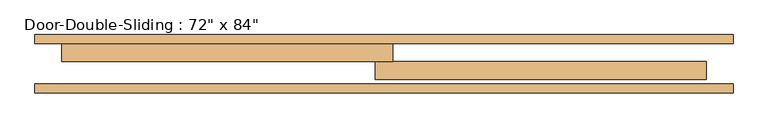
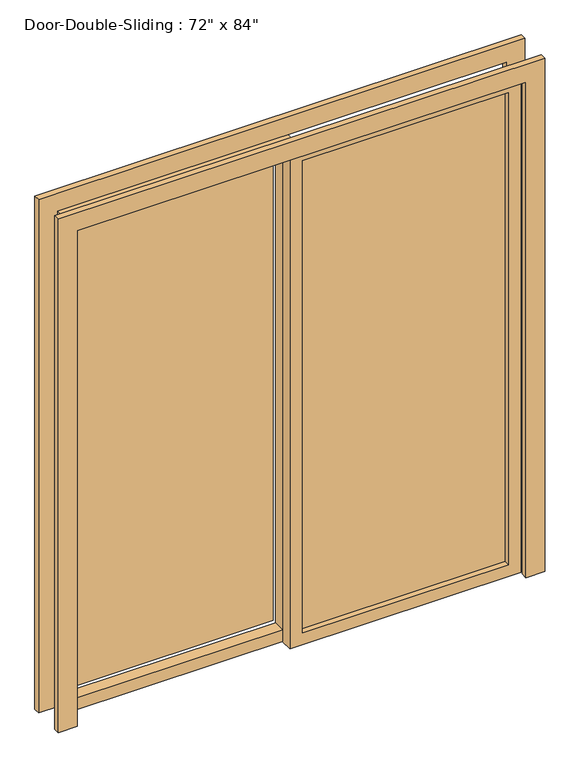
"""IFC4 building model written with IfcOpenShell, lengths in millimetres: door geometry."""

from ifc_helpers import new_model, si_unit, frame, origin, place, context, project, spatial, polyline, outline, extrude, source, transform, mapped, element, save


def door_166d4031(model_context):
    return source(origin(), model_context, "Body", "SweptSolid", [
        extrude(outline(polyline([(0.0, 990.6), (2209.8, 990.6), (2209.8, -990.6), (0.0, -990.6), (0.0, -914.4), (2133.6, -914.4), (2133.6, 914.4), (0.0, 914.4), (0.0, 990.6)])), frame((0.0, 184.15, 0.0), z_axis=(0.0, 1.0, 0.0), x_axis=(0.0, 0.0, 1.0)), (0.0, 0.0, 1.0), 25.4),
        extrude(outline(polyline([(0.0, -990.6), (0.0, -914.4), (2133.6, -914.4), (2133.6, 914.4), (0.0, 914.4), (0.0, 990.6), (2209.8, 990.6), (2209.8, -990.6), (0.0, -990.6)])), frame((0.0, 44.45, 0.0), z_axis=(0.0, 1.0, 0.0), x_axis=(0.0, 0.0, 1.0)), (0.0, 0.0, 1.0), 25.4),
        extrude(outline(polyline([(2133.6, 25.4), (2133.6, -914.4), (0.0, -914.4), (0.0, 25.4), (2133.6, 25.4)]), holes=[polyline([(2082.8, -25.4), (50.8, -25.4), (50.8, -863.6), (2082.8, -863.6), (2082.8, -25.4)])]), frame((0.0, 133.35, 0.0), z_axis=(0.0, 1.0, 0.0), x_axis=(0.0, 0.0, 1.0)), (0.0, 0.0, 1.0), 50.8),
        extrude(outline(polyline([(2133.6, -25.4), (0.0, -25.4), (0.0, 914.4), (2133.6, 914.4), (2133.6, -25.4)]), holes=[polyline([(2082.8, 25.4), (2082.8, 863.6), (50.8, 863.6), (50.8, 25.4), (2082.8, 25.4)])]), frame((0.0, 82.55, 0.0), z_axis=(0.0, 1.0, 0.0), x_axis=(0.0, 0.0, 1.0)), (0.0, 0.0, 1.0), 50.8),
        extrude(outline(polyline([(-25.4, 200.025), (-863.6, 200.025), (-863.6, 206.375), (-25.4, 206.375), (-25.4, 200.025)])), frame((0.0, 0.0, 50.8), z_axis=(0.0, 0.0, 1.0), x_axis=(1.0, 0.0, 0.0)), (0.0, 0.0, 1.0), 2032.0),
        extrude(outline(polyline([(25.4, 111.125), (863.6, 111.125), (863.6, 104.775), (25.4, 104.775), (25.4, 111.125)])), frame((0.0, 0.0, 50.8), z_axis=(0.0, 0.0, 1.0), x_axis=(1.0, 0.0, 0.0)), (0.0, 0.0, 1.0), 2032.0),
    ])


if __name__ == "__main__":
    model = new_model("IFC4")
    model_context = context("Model", 3, world=origin())
    ifc_project = project(units=[si_unit("LENGTHUNIT", "METRE", prefix="MILLI")], contexts=[model_context])
    site = spatial("IfcSite", under=ifc_project)
    building = spatial("IfcBuilding", under=site)
    placement = place(None, origin())
    door_shape = door_166d4031(model_context)
    element("IfcDoor", 1, ObjectType="Door-Double-Sliding : 72\" x 84\"", at=placement, inside=building, context=model_context, shape_type="MappedRepresentation", body=[
        mapped(door_shape, transform((0.0, 0.0, 0.0), x_axis=(1.0, 0.0, 0.0), y_axis=(0.0, 1.0, 0.0), z_axis=(0.0, 0.0, 1.0))),
    ])
    save(model, "model.ifc")

# Revit data of these elements
# Type "Door-Double-Sliding : 72\" x 84\""
#   Type Mark = "9"
#   Construction Type Id = "opn-d45"
#   Assembly Code = "C1020"
#   Analytic Construction = "Wood frame, double glass door "
#   Thickness = 0' - 2"
#   Thermal Resistance (R) = 1.8150 (h·ft²·°F)/BTU
#   Heat Transfer Coefficient (U) = 0.5510 BTU/(h·ft²·°F)
#   Height = 7' - 0"
#   Rail Width = 0' - 2"
#   Stiles = 0' - 2"
#   Trim Projection Ext = 0' - 1"
#   Trim Projection Int = 0' - 1"
#   Trim Width = 0' - 3"
#   Width = 6' - 0"
#   Define Thermal Properties by = 1
#   Glazing = Glass
#   Panel Material = Wood - Birch - Solid Stained Light Low Gloss
#   Trim Material = Paint - Sienna
#   Visual Light Transmittance = 0
#   Solar Heat Gain Coefficient = 0
#   Function = (empty or 0)
#   Wall Closure = (empty or 0)
# Element 1 (IfcDoor, "Door-Double-Sliding : 72\" x 84\"")
#   Materials on its faces: "Paint - Sienna", "Wood - Birch - Solid Stained Light Low Gloss", "Glass"
# Materials
#   "Glass": class "Glass", colour RGB 0 128 192, transparency 0.75, Description = "Soda Lime Glass", Cost = 0
#   "Wood - Birch - Solid Stained Light Low Gloss": class "Wood", colour RGB 210 159 95, transparency 0, Cost = 0
#   "Paint - Sienna": colour RGB 118 70 51, transparency 0, Cost = 0
